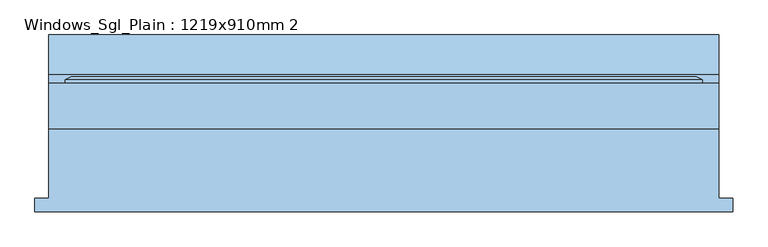
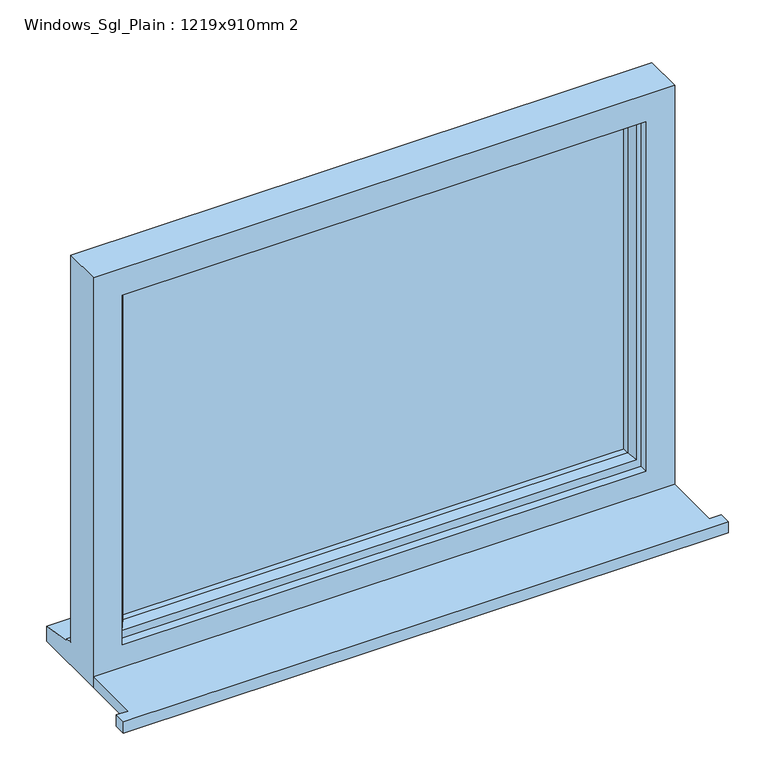
"""IFC4 building model written with IfcOpenShell, lengths in millimetres: window geometry, Windows_Sgl_Plain : 1219x910mm 2."""

from ifc_helpers import new_model, si_unit, frame, origin, place, context, project, spatial, polyline, outline, extrude, faceted_brep, source, transform, mapped, element, save


def windows_sgl_plain_1219x910mm_2_5c67ae2b(model_context):
    return source(origin(), model_context, "Body", "SolidModel", [
        extrude(outline(polyline([(-634.6, -146.0834322), (-634.6, -121.0834322), (-609.6, -121.0834322), (-609.6, 4.9965678), (609.6, 4.9965678), (609.6, -121.0834322), (634.6, -121.0834322), (634.6, -146.0834322), (-634.6, -146.0834322)])), frame((0.0, 0.0, 1200.0), z_axis=(0.0, 0.0, 1.0), x_axis=(1.0, 0.0, 0.0)), (0.0, 0.0, 1.0), 25.0),
        faceted_brep([(-609.6, 4.9965678, 1200.0), (609.6, 4.9965678, 1200.0), (609.6, 4.9965678, 2110.0), (-609.6, 4.9965678, 2110.0), (-549.6, 4.9965678, 2050.0), (549.6, 4.9965678, 2050.0), (549.6, 4.9965678, 1275.0), (-549.6, 4.9965678, 1275.0), (-609.6, 87.9965678, 2110.0), (-609.6, 87.9965678, 1251.0), (-609.6, 102.9965678, 1249.68767), (-609.6, 102.9965678, 1244.7449676), (-609.6, 175.4965678, 1233.8088847), (-609.6, 175.4965678, 1200.0), (609.6, 87.9965678, 2110.0), (609.6, 87.9965678, 1251.0), (-569.6, 87.9965678, 2070.0), (-569.6, 87.9965678, 1263.0), (569.6, 87.9965678, 1263.0), (569.6, 87.9965678, 2070.0), (-569.6, 22.9965678, 2070.0), (-569.6, 22.9965678, 1263.0), (569.6, 22.9965678, 2070.0), (569.6, 22.9965678, 1263.0), (-549.6, 22.9965678, 2050.0), (-549.6, 22.9965678, 1275.0), (549.6, 22.9965678, 1275.0), (549.6, 22.9965678, 2050.0), (609.6, 175.4965678, 1200.0), (609.6, 175.4965678, 1233.8088847), (609.6, 102.9965678, 1244.7449676), (609.6, 102.9965678, 1249.68767)], [[[0, 1, 2, 3], [4, 5, 6, 7]], [[0, 3, 8, 9, 10, 11, 12, 13]], [[9, 8, 14, 15], [16, 17, 18, 19]], [[17, 16, 20, 21]], [[20, 22, 23, 21], [24, 25, 26, 27]], [[24, 4, 7, 25]], [[3, 2, 14, 8]], [[16, 19, 22, 20]], [[5, 4, 24, 27]], [[15, 14, 2, 1, 28, 29, 30, 31]], [[19, 18, 23, 22]], [[5, 27, 26, 6]], [[28, 1, 0, 13]], [[29, 28, 13, 12]], [[30, 29, 12, 11]], [[31, 30, 11, 10]], [[15, 31, 10, 9]], [[21, 23, 18, 17]], [[7, 6, 26, 25]]]),
        extrude(outline(polyline([(539.6, 51.9965678), (-539.6, 51.9965678), (-539.6, 75.9965678), (539.6, 75.9965678), (539.6, 51.9965678)])), frame((0.0, 0.0, 1293.0), z_axis=(0.0, 0.0, 1.0), x_axis=(1.0, 0.0, 0.0)), (0.0, 0.0, 1.0), 747.0),
        faceted_brep([(-579.6, 87.9965678, 2080.0), (-579.6, 93.7700705, 2080.0), (-579.6, 93.7700705, 1253.0), (-579.6, 87.9965678, 1253.0), (-569.6, 22.9965678, 2070.0), (-569.6, 87.9965678, 2070.0), (-569.6, 87.9965678, 1263.0), (-569.6, 22.9965678, 1263.0), (-529.6, 37.4894677, 2030.0), (-539.7480377, 22.9965678, 2040.1480377), (-539.7480377, 22.9965678, 1292.8519623), (-529.6, 37.4894677, 1303.0), (-529.6, 51.9965678, 2030.0), (-529.6, 51.9965678, 1303.0), (-539.6, 75.9965678, 2040.0), (-539.6, 51.9965678, 2040.0), (-539.6, 51.9965678, 1293.0), (-539.6, 75.9965678, 1293.0), (-529.6, 93.7700705, 2030.0), (-529.6, 75.9965678, 2030.0), (-529.6, 75.9965678, 1303.0), (-529.6, 93.7700705, 1303.0), (-547.0457548, 99.5435732, 2047.4457548), (-547.0457548, 99.5435732, 1285.5542452), (-568.8153903, 99.5435732, 2069.2153903), (-568.8153903, 99.5435732, 1263.7846097), (579.6, 93.7700705, 1253.0), (579.6, 87.9965678, 1253.0), (569.6, 87.9965678, 1263.0), (569.6, 22.9965678, 1263.0), (539.7480377, 22.9965678, 1292.8519623), (529.6, 37.4894677, 1303.0), (529.6, 51.9965678, 1303.0), (539.6, 51.9965678, 1293.0), (539.6, 75.9965678, 1293.0), (529.6, 75.9965678, 1303.0), (529.6, 93.7700705, 1303.0), (547.0457548, 99.5435732, 1285.5542452), (568.8153903, 99.5435732, 1263.7846097), (579.6, 93.7700705, 2080.0), (579.6, 87.9965678, 2080.0), (569.6, 87.9965678, 2070.0), (569.6, 22.9965678, 2070.0), (539.7480377, 22.9965678, 2040.1480377), (529.6, 37.4894677, 2030.0), (529.6, 51.9965678, 2030.0), (539.6, 51.9965678, 2040.0), (539.6, 75.9965678, 2040.0), (529.6, 75.9965678, 2030.0), (529.6, 93.7700705, 2030.0), (547.0457548, 99.5435732, 2047.4457548), (568.8153903, 99.5435732, 2069.2153903)], [[[0, 1, 2, 3]], [[4, 5, 6, 7]], [[8, 9, 10, 11]], [[12, 8, 11, 13]], [[14, 15, 16, 17]], [[18, 19, 20, 21]], [[22, 18, 21, 23]], [[1, 24, 25, 2]], [[3, 2, 26, 27]], [[7, 6, 28, 29]], [[11, 10, 30, 31]], [[13, 11, 31, 32]], [[17, 16, 33, 34]], [[21, 20, 35, 36]], [[23, 21, 36, 37]], [[2, 25, 38, 26]], [[27, 26, 39, 40]], [[29, 28, 41, 42]], [[31, 30, 43, 44]], [[32, 31, 44, 45]], [[34, 33, 46, 47]], [[36, 35, 48, 49]], [[37, 36, 49, 50]], [[26, 38, 51, 39]], [[40, 39, 1, 0]], [[3, 27, 40, 0], [5, 41, 28, 6]], [[42, 41, 5, 4]], [[7, 29, 42, 4], [9, 43, 30, 10]], [[44, 43, 9, 8]], [[45, 44, 8, 12]], [[15, 46, 33, 16], [13, 32, 45, 12]], [[47, 46, 15, 14]], [[17, 34, 47, 14], [19, 48, 35, 20]], [[49, 48, 19, 18]], [[50, 49, 18, 22]], [[24, 51, 38, 25], [23, 37, 50, 22]], [[39, 51, 24, 1]]]),
    ])


if __name__ == "__main__":
    model = new_model("IFC4")
    model_context = context("Model", 3, world=origin())
    ifc_project = project(units=[si_unit("LENGTHUNIT", "METRE", prefix="MILLI")], contexts=[model_context])
    site = spatial("IfcSite", under=ifc_project)
    building = spatial("IfcBuilding", under=site)
    placement = place(None, origin())
    windows_sgl_plain_1219x910mm_2_shape = windows_sgl_plain_1219x910mm_2_5c67ae2b(model_context)
    element("IfcWindow", 1, ObjectType="Windows_Sgl_Plain : 1219x910mm 2", at=placement, inside=building, context=model_context, shape_type="MappedRepresentation", body=[
        mapped(windows_sgl_plain_1219x910mm_2_shape, transform((0.0, 0.0, 0.0), x_axis=(1.0, 0.0, 0.0), y_axis=(0.0, 1.0, 0.0), z_axis=(0.0, 0.0, 1.0))),
    ])
    save(model, "model.ifc")

# Revit data of these elements
# Type "Windows_Sgl_Plain : 1219x910mm 2"
#   Type Mark = "61"
#   Operation = "SinglePanel"
#   Construction Type Id = "SGL"
#   Manufacturer = "Revit"
#   Keynote = "L10"
#   Analytic Construction = "Large single-glazed windows"
#   Wrap Layers (Ext) from Ext = 0.336286 ft
#   Wrap Layers (Int) from Ext = 0.582349 ft
#   Window Board Projection = 0.082021 ft
#   Window Board Extension = 0.082021 ft
#   Visual Light Transmittance = 0.9
#   Solar Heat Gain Coefficient = 0.86
#   Rough Width = 4.0 ft
#   Rough Height = 2.985564 ft
#   Height = 2.985564 ft
#   Width = 4.0 ft
#   Heat Transfer Coefficient (U) = 5.5617 W/(m²·K)
#   Glazing Thickness = 0.07874 ft
#   FrameOffset - External = 0.164042 ft
#   Frame Depth = 0.213255 ft
#   Default Head Height = 6.922572 ft
#   Cill Depth = 0.287073 ft
#   Cavity Closer Width = 0.164042 ft
#   Cavity Closer Offset from Ext = 0.336286 ft
#   Cavity Closer Depth = 0.278871 ft
#   Vis - Cavity Closers = yes
#   Define Thermal Properties by = 1
#   Material Trim = Window Frame
#   Material Glass = Glass
#   Material Frame = Window Frame
#   Wall Closure = (empty or 0)
# Element 1 (IfcWindow, "Windows_Sgl_Plain : 1219x910mm 2")
#   Materials on its faces: "Window Frame", "Glass"
# Materials
#   "Window Frame": colour RGB 249 249 249, transparency 0, Keynote = "L10", Cost = 0
#   "Glass": class "Glass", colour RGB 0 128 192, transparency 0.9, Description = "Soda Lime Glass", Cost = 0
